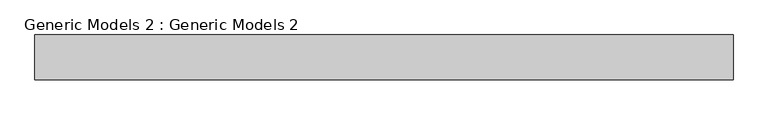
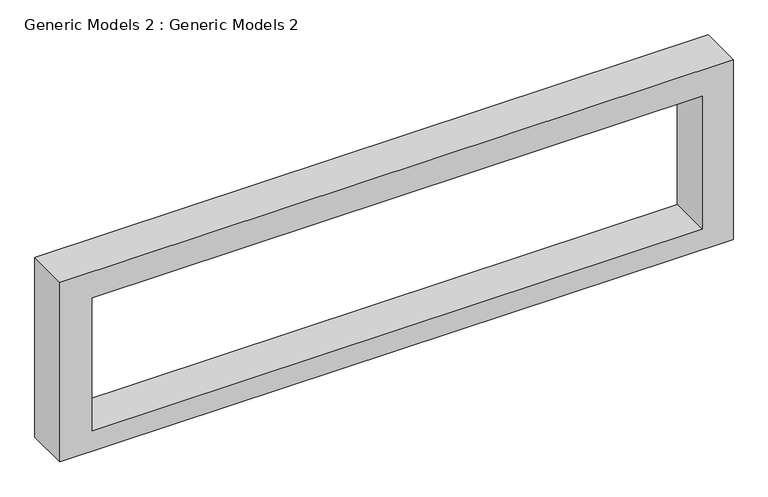
"""IFC4 building model written with IfcOpenShell, lengths in millimetres: proxy geometry, Generic Models 2 : Generic Models 2."""

from ifc_helpers import new_model, si_unit, frame, origin, place, context, project, spatial, polyline, outline, extrude, source, transform, mapped, element, save


def generic_models_2_generic_models_2_98d93cec(model_context):
    return source(origin(), model_context, "Body", "SweptSolid", [
        extrude(outline(polyline([(1542.0723341, 4365.8975541), (1542.0723341, -370.8055709), (204.5269001, -370.8055709), (204.5269001, 4365.8975541), (1542.0723341, 4365.8975541)]), holes=[polyline([(1346.7321748, 4149.7924066), (356.1321748, 4149.7924066), (356.1321748, -142.8075934), (1346.7321748, -142.8075934), (1346.7321748, 4149.7924066)])]), frame((0.0, -7272.3064015, 0.0), z_axis=(0.0, 1.0, 0.0), x_axis=(0.0, 0.0, 1.0)), (0.0, 0.0, 1.0), 304.8),
    ])


if __name__ == "__main__":
    model = new_model("IFC4")
    model_context = context("Model", 3, world=origin())
    ifc_project = project(units=[si_unit("LENGTHUNIT", "METRE", prefix="MILLI")], contexts=[model_context])
    site = spatial("IfcSite", under=ifc_project)
    building = spatial("IfcBuilding", under=site)
    placement = place(None, origin())
    generic_models_2_generic_models_2_shape = generic_models_2_generic_models_2_98d93cec(model_context)
    element("IfcBuildingElementProxy", 1, Name="Generic Models 2 : Generic Models 2", ObjectType="Generic Models 2 : Generic Models 2", at=placement, inside=building, context=model_context, shape_type="MappedRepresentation", body=[
        mapped(generic_models_2_generic_models_2_shape, transform((0.0, 0.0, 0.0), x_axis=(1.0, 0.0, 0.0), y_axis=(0.0, 1.0, 0.0), z_axis=(0.0, 0.0, 1.0))),
    ])
    save(model, "model.ifc")

# Revit data of these elements
# Element 1 (IfcBuildingElementProxy, "Generic Models 2 : Generic Models 2")
#   Materials on its faces: "Parking Stripe"
# Materials
#   "Parking Stripe": class "Paint", colour RGB 250 250 91, transparency 0, Cost = 0
